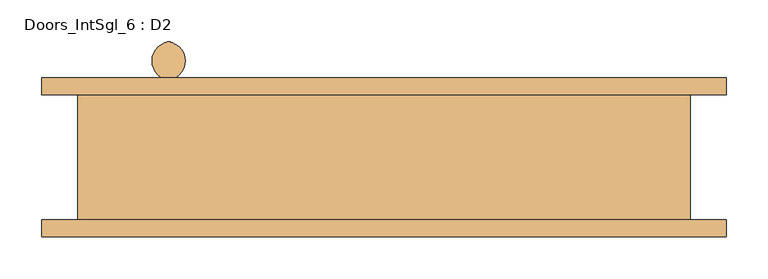
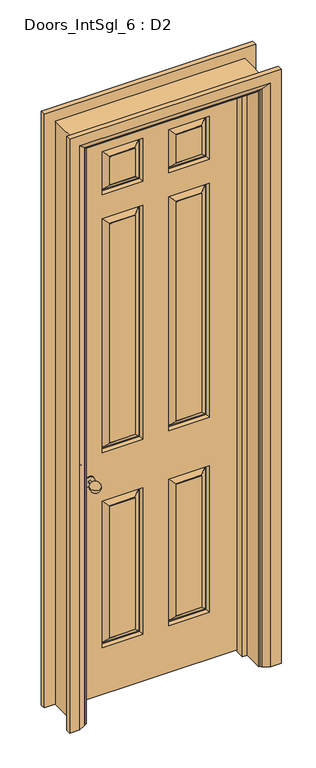
"""IFC4 building model written with IfcOpenShell, lengths in millimetres: door geometry, Doors_IntSgl_6 : D2."""

from ifc_helpers import new_model, si_unit, point, frame, origin, place, context, project, spatial, polyline, circle_curve, ellipse_curve, trimmed, outline, extrude, faceted_brep, source, transform, mapped, element, save
from ifc_brep_helpers import plane_surface, cylinder_surface, revolved_surface, advanced_brep


def doors_intsgl_6_d2_b603f254(model_context):
    return source(origin(), model_context, "Body", "SolidModel", [
        advanced_brep(
        [(-253.0, 18.0, 900.0), (-258.0, -26.437411, 900.0), (-263.0, 18.0, 900.0), (-263.0, 33.0, 900.0), (-253.0, 33.0, 900.0), (-278.0, 37.0, 900.0), (-238.0, 37.0, 900.0), (-278.0, 33.0, 900.0), (-238.0, 33.0, 900.0)],
        [
            (0, 1, circle_curve(frame((-261.1884862, -3.5786495, 900.0), z_axis=(0.0, 0.0, -1.0), x_axis=(0.0, 1.0, 0.0)), 23.0800654)),
            (1, 2, circle_curve(frame((-254.8115138, -3.5786495, 900.0), z_axis=(0.0, 0.0, -1.0), x_axis=(0.0, 1.0, 0.0)), 23.0800654)),
            (2, 0, circle_curve(frame((-258.0, 18.0, 900.0), z_axis=(0.0, -1.0, 0.0), x_axis=(-1.0, 0.0, 0.0)), 5.0)),
            (0, 2, circle_curve(frame((-258.0, 18.0, 900.0), z_axis=(0.0, -1.0, 0.0), x_axis=(-1.0, 0.0, 0.0)), 5.0)),
            (2, 3),
            (3, 4, circle_curve(frame((-258.0, 33.0, 900.0), z_axis=(0.0, -1.0, 0.0), x_axis=(-1.0, 0.0, 0.0)), 5.0)),
            (4, 0),
            (4, 3, circle_curve(frame((-258.0, 33.0, 900.0), z_axis=(0.0, -1.0, 0.0), x_axis=(-1.0, 0.0, 0.0)), 5.0)),
            (5, 6, circle_curve(frame((-258.0, 37.0, 900.0), z_axis=(0.0, 1.0, 0.0), x_axis=(1.0, 0.0, 0.0)), 20.0)),
            (6, 5, circle_curve(frame((-258.0, 37.0, 900.0), z_axis=(0.0, 1.0, 0.0), x_axis=(1.0, 0.0, 0.0)), 20.0)),
            (7, 8, circle_curve(frame((-258.0, 33.0, 900.0), z_axis=(0.0, -1.0, 0.0), x_axis=(1.0, 0.0, 0.0)), 20.0)),
            (8, 7, circle_curve(frame((-258.0, 33.0, 900.0), z_axis=(0.0, -1.0, 0.0), x_axis=(1.0, 0.0, 0.0)), 20.0)),
            (6, 8),
            (7, 5),
        ],
        [
            revolved_surface(trimmed(ellipse_curve(frame((-254.8115138, -3.5786495, 900.0), z_axis=(0.0, 0.0, -1.0), x_axis=(0.0, 1.0, 0.0)), 23.0800654, 23.0800654), [point((-258.0, -26.437411, 900.0))], [point((-263.0, 18.0, 900.0))], True, "CARTESIAN"), (-258.0, 33.0, 900.0), (0.0, 1.0, 0.0)),
            cylinder_surface(frame((-258.0, 33.0, 900.0), z_axis=(0.0, 1.0, 0.0), x_axis=(-1.0, 0.0, 0.0)), 5.0),
            plane_surface(frame((-238.0, 37.0, 900.0), z_axis=(0.0, 1.0, 0.0), x_axis=(0.0, 0.0, 1.0))),
            plane_surface(frame((-238.0, 33.0, 900.0), z_axis=(0.0, -1.0, 0.0), x_axis=(0.0, 0.0, -1.0))),
            cylinder_surface(frame((-258.0, 33.0, 900.0), z_axis=(0.0, 1.0, 0.0), x_axis=(1.0, 0.0, 0.0)), 20.0),
        ],
        [
            (0, [[1, 2, 3]]),
            (0, [[-1, 4, -2]]),
            (1, [[5, 6, 7, -3]]),
            (1, [[-7, 8, -5, -4]]),
            (2, [[9, 10]]),
            (3, [[11, 12], [-8, -6]]),
            (4, [[13, -11, 14, -10]]),
            (4, [[-14, -12, -13, -9]]),
        ],
    ),
        advanced_brep(
        [(-253.0, 94.0, 900.0), (-263.0, 94.0, 900.0), (-258.0, 138.437411, 900.0), (-253.0, 79.0, 900.0), (-263.0, 79.0, 900.0), (-278.0, 75.0, 900.0), (-238.0, 75.0, 900.0), (-278.0, 79.0, 900.0), (-238.0, 79.0, 900.0)],
        [
            (0, 1, circle_curve(frame((-258.0, 94.0, 900.0), z_axis=(0.0, 1.0, 0.0), x_axis=(-1.0, 0.0, 0.0)), 5.0)),
            (1, 2, circle_curve(frame((-254.8115138, 115.5786495, 900.0), z_axis=(0.0, 0.0, -1.0), x_axis=(0.0, -1.0, 0.0)), 23.0800654)),
            (2, 0, circle_curve(frame((-261.1884862, 115.5786495, 900.0), z_axis=(0.0, 0.0, -1.0), x_axis=(0.0, -1.0, 0.0)), 23.0800654)),
            (1, 0, circle_curve(frame((-258.0, 94.0, 900.0), z_axis=(0.0, 1.0, 0.0), x_axis=(-1.0, 0.0, 0.0)), 5.0)),
            (0, 3),
            (3, 4, circle_curve(frame((-258.0, 79.0, 900.0), z_axis=(0.0, 1.0, 0.0), x_axis=(-1.0, 0.0, 0.0)), 5.0)),
            (4, 1),
            (4, 3, circle_curve(frame((-258.0, 79.0, 900.0), z_axis=(0.0, 1.0, 0.0), x_axis=(-1.0, 0.0, 0.0)), 5.0)),
            (5, 6, circle_curve(frame((-258.0, 75.0, 900.0), z_axis=(0.0, -1.0, 0.0), x_axis=(1.0, 0.0, 0.0)), 20.0)),
            (6, 5, circle_curve(frame((-258.0, 75.0, 900.0), z_axis=(0.0, -1.0, 0.0), x_axis=(1.0, 0.0, 0.0)), 20.0)),
            (7, 8, circle_curve(frame((-258.0, 79.0, 900.0), z_axis=(0.0, 1.0, 0.0), x_axis=(1.0, 0.0, 0.0)), 20.0)),
            (8, 7, circle_curve(frame((-258.0, 79.0, 900.0), z_axis=(0.0, 1.0, 0.0), x_axis=(1.0, 0.0, 0.0)), 20.0)),
            (5, 7),
            (8, 6),
        ],
        [
            revolved_surface(trimmed(ellipse_curve(frame((-254.8115138, 115.5786495, 900.0), z_axis=(0.0, 0.0, 1.0), x_axis=(0.0, -1.0, 0.0)), 23.0800654, 23.0800654), [point((-258.0, 138.437411, 900.0))], [point((-263.0, 94.0, 900.0))], True, "CARTESIAN"), (-258.0, 79.0, 900.0), (0.0, -1.0, 0.0)),
            cylinder_surface(frame((-258.0, 79.0, 900.0), z_axis=(0.0, -1.0, 0.0), x_axis=(-1.0, 0.0, 0.0)), 5.0),
            plane_surface(frame((-238.0, 75.0, 900.0), z_axis=(0.0, -1.0, 0.0), x_axis=(0.0, 0.0, 1.0))),
            plane_surface(frame((-238.0, 79.0, 900.0), z_axis=(0.0, 1.0, 0.0), x_axis=(0.0, 0.0, -1.0))),
            cylinder_surface(frame((-258.0, 79.0, 900.0), z_axis=(0.0, -1.0, 0.0), x_axis=(1.0, 0.0, 0.0)), 20.0),
        ],
        [
            (0, [[1, 2, 3]]),
            (0, [[-2, 4, -3]]),
            (1, [[-1, 5, 6, 7]]),
            (1, [[-4, -7, 8, -5]]),
            (2, [[9, 10]]),
            (3, [[11, 12], [-6, -8]]),
            (4, [[-9, 13, -12, 14]]),
            (4, [[-10, -14, -11, -13]]),
        ],
    ),
        faceted_brep([(-333.0, 37.0, 2358.0), (-333.0, 37.0, 8.0), (333.0, 37.0, 8.0), (333.0, 37.0, 2358.0), (-50.0, 37.0, 800.0), (-50.0, 37.0, 200.0), (-208.0, 37.0, 200.0), (-208.0, 37.0, 800.0), (208.0, 37.0, 800.0), (208.0, 37.0, 200.0), (50.0, 37.0, 200.0), (50.0, 37.0, 800.0), (-50.0, 37.0, 1958.0), (-50.0, 37.0, 1000.0), (-208.0, 37.0, 1000.0), (-208.0, 37.0, 1958.0), (208.0, 37.0, 1958.0), (208.0, 37.0, 1000.0), (50.0, 37.0, 1000.0), (50.0, 37.0, 1958.0), (-50.0, 37.0, 2233.0), (-50.0, 37.0, 2058.0), (-208.0, 37.0, 2058.0), (-208.0, 37.0, 2233.0), (208.0, 37.0, 2233.0), (208.0, 37.0, 2058.0), (50.0, 37.0, 2058.0), (50.0, 37.0, 2233.0), (-80.0, 37.0, 230.0), (-80.0, 37.0, 770.0), (-178.0, 37.0, 770.0), (-178.0, 37.0, 230.0), (178.0, 37.0, 230.0), (178.0, 37.0, 770.0), (80.0, 37.0, 770.0), (80.0, 37.0, 230.0), (-80.0, 37.0, 1030.0), (-80.0, 37.0, 1928.0), (-178.0, 37.0, 1928.0), (-178.0, 37.0, 1030.0), (178.0, 37.0, 1030.0), (178.0, 37.0, 1928.0), (80.0, 37.0, 1928.0), (80.0, 37.0, 1030.0), (-80.0, 37.0, 2088.0), (-80.0, 37.0, 2203.0), (-178.0, 37.0, 2203.0), (-178.0, 37.0, 2088.0), (178.0, 37.0, 2088.0), (178.0, 37.0, 2203.0), (80.0, 37.0, 2203.0), (80.0, 37.0, 2088.0), (-333.0, 75.0, 2358.0), (333.0, 75.0, 2358.0), (333.0, 75.0, 8.0), (-333.0, 75.0, 8.0), (50.0, 75.0, 800.0), (50.0, 75.0, 200.0), (208.0, 75.0, 200.0), (208.0, 75.0, 800.0), (-208.0, 75.0, 800.0), (-208.0, 75.0, 200.0), (-50.0, 75.0, 200.0), (-50.0, 75.0, 800.0), (50.0, 75.0, 1958.0), (50.0, 75.0, 1000.0), (208.0, 75.0, 1000.0), (208.0, 75.0, 1958.0), (-208.0, 75.0, 1958.0), (-208.0, 75.0, 1000.0), (-50.0, 75.0, 1000.0), (-50.0, 75.0, 1958.0), (50.0, 75.0, 2233.0), (50.0, 75.0, 2058.0), (208.0, 75.0, 2058.0), (208.0, 75.0, 2233.0), (-208.0, 75.0, 2233.0), (-208.0, 75.0, 2058.0), (-50.0, 75.0, 2058.0), (-50.0, 75.0, 2233.0), (80.0, 75.0, 230.0), (80.0, 75.0, 770.0), (178.0, 75.0, 770.0), (178.0, 75.0, 230.0), (-178.0, 75.0, 230.0), (-178.0, 75.0, 770.0), (-80.0, 75.0, 770.0), (-80.0, 75.0, 230.0), (80.0, 75.0, 1030.0), (80.0, 75.0, 1928.0), (178.0, 75.0, 1928.0), (178.0, 75.0, 1030.0), (-178.0, 75.0, 1030.0), (-178.0, 75.0, 1928.0), (-80.0, 75.0, 1928.0), (-80.0, 75.0, 1030.0), (80.0, 75.0, 2088.0), (80.0, 75.0, 2203.0), (178.0, 75.0, 2203.0), (178.0, 75.0, 2088.0), (-178.0, 75.0, 2088.0), (-178.0, 75.0, 2203.0), (-80.0, 75.0, 2203.0), (-80.0, 75.0, 2088.0), (80.0, 74.0, 230.0), (80.0, 74.0, 770.0), (58.0, 60.0, 208.0), (58.0, 60.0, 792.0), (78.0, 74.0, 772.0), (78.0, 74.0, 228.0), (53.0, 60.0, 797.0), (53.0, 60.0, 203.0), (178.0, 74.0, 770.0), (200.0, 60.0, 792.0), (180.0, 74.0, 772.0), (205.0, 60.0, 797.0), (178.0, 74.0, 230.0), (200.0, 60.0, 208.0), (180.0, 74.0, 228.0), (205.0, 60.0, 203.0), (-178.0, 74.0, 230.0), (-178.0, 74.0, 770.0), (-200.0, 60.0, 208.0), (-200.0, 60.0, 792.0), (-180.0, 74.0, 772.0), (-180.0, 74.0, 228.0), (-205.0, 60.0, 797.0), (-205.0, 60.0, 203.0), (-80.0, 74.0, 770.0), (-58.0, 60.0, 792.0), (-78.0, 74.0, 772.0), (-53.0, 60.0, 797.0), (-80.0, 74.0, 230.0), (-58.0, 60.0, 208.0), (-78.0, 74.0, 228.0), (-53.0, 60.0, 203.0), (80.0, 74.0, 1030.0), (80.0, 74.0, 1928.0), (58.0, 60.0, 1008.0), (58.0, 60.0, 1950.0), (78.0, 74.0, 1930.0), (78.0, 74.0, 1028.0), (53.0, 60.0, 1955.0), (53.0, 60.0, 1003.0), (178.0, 74.0, 1928.0), (200.0, 60.0, 1950.0), (180.0, 74.0, 1930.0), (205.0, 60.0, 1955.0), (178.0, 74.0, 1030.0), (200.0, 60.0, 1008.0), (180.0, 74.0, 1028.0), (205.0, 60.0, 1003.0), (-178.0, 74.0, 1030.0), (-178.0, 74.0, 1928.0), (-200.0, 60.0, 1008.0), (-200.0, 60.0, 1950.0), (-180.0, 74.0, 1930.0), (-180.0, 74.0, 1028.0), (-205.0, 60.0, 1955.0), (-205.0, 60.0, 1003.0), (-80.0, 74.0, 1928.0), (-58.0, 60.0, 1950.0), (-78.0, 74.0, 1930.0), (-53.0, 60.0, 1955.0), (-80.0, 74.0, 1030.0), (-58.0, 60.0, 1008.0), (-78.0, 74.0, 1028.0), (-53.0, 60.0, 1003.0), (80.0, 74.0, 2088.0), (80.0, 74.0, 2203.0), (58.0, 60.0, 2066.0), (58.0, 60.0, 2225.0), (78.0, 74.0, 2205.0), (78.0, 74.0, 2086.0), (53.0, 60.0, 2230.0), (53.0, 60.0, 2061.0), (178.0, 74.0, 2203.0), (200.0, 60.0, 2225.0), (180.0, 74.0, 2205.0), (205.0, 60.0, 2230.0), (178.0, 74.0, 2088.0), (200.0, 60.0, 2066.0), (180.0, 74.0, 2086.0), (205.0, 60.0, 2061.0), (-178.0, 74.0, 2088.0), (-178.0, 74.0, 2203.0), (-200.0, 60.0, 2066.0), (-200.0, 60.0, 2225.0), (-180.0, 74.0, 2205.0), (-180.0, 74.0, 2086.0), (-205.0, 60.0, 2230.0), (-205.0, 60.0, 2061.0), (-80.0, 74.0, 2203.0), (-58.0, 60.0, 2225.0), (-78.0, 74.0, 2205.0), (-53.0, 60.0, 2230.0), (-80.0, 74.0, 2088.0), (-58.0, 60.0, 2066.0), (-78.0, 74.0, 2086.0), (-53.0, 60.0, 2061.0), (-80.0, 38.0, 230.0), (-80.0, 38.0, 770.0), (-58.0, 52.0, 208.0), (-58.0, 52.0, 792.0), (-78.0, 38.0, 772.0), (-78.0, 38.0, 228.0), (-53.0, 52.0, 797.0), (-53.0, 52.0, 203.0), (-178.0, 38.0, 770.0), (-200.0, 52.0, 792.0), (-180.0, 38.0, 772.0), (-205.0, 52.0, 797.0), (-178.0, 38.0, 230.0), (-200.0, 52.0, 208.0), (-180.0, 38.0, 228.0), (-205.0, 52.0, 203.0), (178.0, 38.0, 230.0), (178.0, 38.0, 770.0), (200.0, 52.0, 208.0), (200.0, 52.0, 792.0), (180.0, 38.0, 772.0), (180.0, 38.0, 228.0), (205.0, 52.0, 797.0), (205.0, 52.0, 203.0), (80.0, 38.0, 770.0), (58.0, 52.0, 792.0), (78.0, 38.0, 772.0), (53.0, 52.0, 797.0), (80.0, 38.0, 230.0), (58.0, 52.0, 208.0), (78.0, 38.0, 228.0), (53.0, 52.0, 203.0), (-80.0, 38.0, 1030.0), (-80.0, 38.0, 1928.0), (-58.0, 52.0, 1008.0), (-58.0, 52.0, 1950.0), (-78.0, 38.0, 1930.0), (-78.0, 38.0, 1028.0), (-53.0, 52.0, 1955.0), (-53.0, 52.0, 1003.0), (-178.0, 38.0, 1928.0), (-200.0, 52.0, 1950.0), (-180.0, 38.0, 1930.0), (-205.0, 52.0, 1955.0), (-178.0, 38.0, 1030.0), (-200.0, 52.0, 1008.0), (-180.0, 38.0, 1028.0), (-205.0, 52.0, 1003.0), (178.0, 38.0, 1030.0), (178.0, 38.0, 1928.0), (200.0, 52.0, 1008.0), (200.0, 52.0, 1950.0), (180.0, 38.0, 1930.0), (180.0, 38.0, 1028.0), (205.0, 52.0, 1955.0), (205.0, 52.0, 1003.0), (80.0, 38.0, 1928.0), (58.0, 52.0, 1950.0), (78.0, 38.0, 1930.0), (53.0, 52.0, 1955.0), (80.0, 38.0, 1030.0), (58.0, 52.0, 1008.0), (78.0, 38.0, 1028.0), (53.0, 52.0, 1003.0), (-80.0, 38.0, 2088.0), (-80.0, 38.0, 2203.0), (-58.0, 52.0, 2066.0), (-58.0, 52.0, 2225.0), (-78.0, 38.0, 2205.0), (-78.0, 38.0, 2086.0), (-53.0, 52.0, 2230.0), (-53.0, 52.0, 2061.0), (-178.0, 38.0, 2203.0), (-200.0, 52.0, 2225.0), (-180.0, 38.0, 2205.0), (-205.0, 52.0, 2230.0), (-178.0, 38.0, 2088.0), (-200.0, 52.0, 2066.0), (-180.0, 38.0, 2086.0), (-205.0, 52.0, 2061.0), (178.0, 38.0, 2088.0), (178.0, 38.0, 2203.0), (200.0, 52.0, 2066.0), (200.0, 52.0, 2225.0), (180.0, 38.0, 2205.0), (180.0, 38.0, 2086.0), (205.0, 52.0, 2230.0), (205.0, 52.0, 2061.0), (80.0, 38.0, 2203.0), (58.0, 52.0, 2225.0), (78.0, 38.0, 2205.0), (53.0, 52.0, 2230.0), (80.0, 38.0, 2088.0), (58.0, 52.0, 2066.0), (78.0, 38.0, 2086.0), (53.0, 52.0, 2061.0)], [[[0, 1, 2, 3], [4, 5, 6, 7], [8, 9, 10, 11], [12, 13, 14, 15], [16, 17, 18, 19], [20, 21, 22, 23], [24, 25, 26, 27]], [[28, 29, 30, 31]], [[32, 33, 34, 35]], [[36, 37, 38, 39]], [[40, 41, 42, 43]], [[44, 45, 46, 47]], [[48, 49, 50, 51]], [[52, 53, 54, 55], [56, 57, 58, 59], [60, 61, 62, 63], [64, 65, 66, 67], [68, 69, 70, 71], [72, 73, 74, 75], [76, 77, 78, 79]], [[80, 81, 82, 83]], [[84, 85, 86, 87]], [[88, 89, 90, 91]], [[92, 93, 94, 95]], [[96, 97, 98, 99]], [[100, 101, 102, 103]], [[1, 0, 52, 55]], [[2, 1, 55, 54]], [[3, 2, 54, 53]], [[0, 3, 53, 52]], [[104, 105, 81, 80]], [[106, 107, 108, 109]], [[56, 110, 111, 57]], [[81, 105, 112, 82]], [[108, 107, 113, 114]], [[110, 56, 59, 115]], [[82, 112, 116, 83]], [[114, 113, 117, 118]], [[115, 59, 58, 119]], [[104, 80, 83, 116]], [[109, 108, 114, 118], [105, 104, 116, 112]], [[106, 109, 118, 117]], [[111, 110, 115, 119], [107, 106, 117, 113]], [[57, 111, 119, 58]], [[120, 121, 85, 84]], [[122, 123, 124, 125]], [[60, 126, 127, 61]], [[85, 121, 128, 86]], [[124, 123, 129, 130]], [[126, 60, 63, 131]], [[86, 128, 132, 87]], [[130, 129, 133, 134]], [[131, 63, 62, 135]], [[120, 84, 87, 132]], [[125, 124, 130, 134], [121, 120, 132, 128]], [[122, 125, 134, 133]], [[127, 126, 131, 135], [123, 122, 133, 129]], [[61, 127, 135, 62]], [[136, 137, 89, 88]], [[138, 139, 140, 141]], [[64, 142, 143, 65]], [[89, 137, 144, 90]], [[140, 139, 145, 146]], [[142, 64, 67, 147]], [[90, 144, 148, 91]], [[146, 145, 149, 150]], [[147, 67, 66, 151]], [[136, 88, 91, 148]], [[141, 140, 146, 150], [137, 136, 148, 144]], [[138, 141, 150, 149]], [[143, 142, 147, 151], [139, 138, 149, 145]], [[65, 143, 151, 66]], [[152, 153, 93, 92]], [[154, 155, 156, 157]], [[68, 158, 159, 69]], [[93, 153, 160, 94]], [[156, 155, 161, 162]], [[158, 68, 71, 163]], [[94, 160, 164, 95]], [[162, 161, 165, 166]], [[163, 71, 70, 167]], [[152, 92, 95, 164]], [[157, 156, 162, 166], [153, 152, 164, 160]], [[154, 157, 166, 165]], [[159, 158, 163, 167], [155, 154, 165, 161]], [[69, 159, 167, 70]], [[168, 169, 97, 96]], [[170, 171, 172, 173]], [[72, 174, 175, 73]], [[97, 169, 176, 98]], [[172, 171, 177, 178]], [[174, 72, 75, 179]], [[98, 176, 180, 99]], [[178, 177, 181, 182]], [[179, 75, 74, 183]], [[168, 96, 99, 180]], [[173, 172, 178, 182], [169, 168, 180, 176]], [[170, 173, 182, 181]], [[175, 174, 179, 183], [171, 170, 181, 177]], [[73, 175, 183, 74]], [[184, 185, 101, 100]], [[186, 187, 188, 189]], [[76, 190, 191, 77]], [[101, 185, 192, 102]], [[188, 187, 193, 194]], [[190, 76, 79, 195]], [[102, 192, 196, 103]], [[194, 193, 197, 198]], [[195, 79, 78, 199]], [[184, 100, 103, 196]], [[189, 188, 194, 198], [185, 184, 196, 192]], [[186, 189, 198, 197]], [[191, 190, 195, 199], [187, 186, 197, 193]], [[77, 191, 199, 78]], [[200, 201, 29, 28]], [[202, 203, 204, 205]], [[4, 206, 207, 5]], [[29, 201, 208, 30]], [[204, 203, 209, 210]], [[206, 4, 7, 211]], [[30, 208, 212, 31]], [[210, 209, 213, 214]], [[211, 7, 6, 215]], [[200, 28, 31, 212]], [[205, 204, 210, 214], [201, 200, 212, 208]], [[202, 205, 214, 213]], [[207, 206, 211, 215], [203, 202, 213, 209]], [[5, 207, 215, 6]], [[216, 217, 33, 32]], [[218, 219, 220, 221]], [[8, 222, 223, 9]], [[33, 217, 224, 34]], [[220, 219, 225, 226]], [[222, 8, 11, 227]], [[34, 224, 228, 35]], [[226, 225, 229, 230]], [[227, 11, 10, 231]], [[216, 32, 35, 228]], [[221, 220, 226, 230], [217, 216, 228, 224]], [[218, 221, 230, 229]], [[223, 222, 227, 231], [219, 218, 229, 225]], [[9, 223, 231, 10]], [[232, 233, 37, 36]], [[234, 235, 236, 237]], [[12, 238, 239, 13]], [[37, 233, 240, 38]], [[236, 235, 241, 242]], [[238, 12, 15, 243]], [[38, 240, 244, 39]], [[242, 241, 245, 246]], [[243, 15, 14, 247]], [[232, 36, 39, 244]], [[237, 236, 242, 246], [233, 232, 244, 240]], [[234, 237, 246, 245]], [[239, 238, 243, 247], [235, 234, 245, 241]], [[13, 239, 247, 14]], [[248, 249, 41, 40]], [[250, 251, 252, 253]], [[16, 254, 255, 17]], [[41, 249, 256, 42]], [[252, 251, 257, 258]], [[254, 16, 19, 259]], [[42, 256, 260, 43]], [[258, 257, 261, 262]], [[259, 19, 18, 263]], [[248, 40, 43, 260]], [[253, 252, 258, 262], [249, 248, 260, 256]], [[250, 253, 262, 261]], [[255, 254, 259, 263], [251, 250, 261, 257]], [[17, 255, 263, 18]], [[264, 265, 45, 44]], [[266, 267, 268, 269]], [[20, 270, 271, 21]], [[45, 265, 272, 46]], [[268, 267, 273, 274]], [[270, 20, 23, 275]], [[46, 272, 276, 47]], [[274, 273, 277, 278]], [[275, 23, 22, 279]], [[264, 44, 47, 276]], [[269, 268, 274, 278], [265, 264, 276, 272]], [[266, 269, 278, 277]], [[271, 270, 275, 279], [267, 266, 277, 273]], [[21, 271, 279, 22]], [[280, 281, 49, 48]], [[282, 283, 284, 285]], [[24, 286, 287, 25]], [[49, 281, 288, 50]], [[284, 283, 289, 290]], [[286, 24, 27, 291]], [[50, 288, 292, 51]], [[290, 289, 293, 294]], [[291, 27, 26, 295]], [[280, 48, 51, 292]], [[285, 284, 290, 294], [281, 280, 292, 288]], [[282, 285, 294, 293]], [[287, 286, 291, 295], [283, 282, 293, 289]], [[25, 287, 295, 26]]]),
        faceted_brep([(-335.0, 75.0, 0.0), (-335.0, -75.0, 0.0), (-367.0, -75.0, 0.0), (-367.0, 75.0, 0.0), (-335.0, 75.0, 2360.0), (-335.0, -75.0, 2360.0), (-367.0, -75.0, 2392.0), (-367.0, 75.0, 2392.0), (335.0, 75.0, 0.0), (367.0, 75.0, 0.0), (367.0, -75.0, 0.0), (335.0, -75.0, 0.0), (335.0, 75.0, 2360.0), (367.0, 75.0, 2392.0), (367.0, -75.0, 2392.0), (335.0, -75.0, 2360.0)], [[[0, 1, 2, 3]], [[1, 0, 4, 5]], [[2, 1, 5, 6]], [[3, 2, 6, 7]], [[0, 3, 7, 4]], [[8, 9, 10, 11]], [[12, 13, 9, 8]], [[13, 14, 10, 9]], [[14, 15, 11, 10]], [[15, 12, 8, 11]], [[5, 4, 12, 15]], [[6, 5, 15, 14]], [[7, 6, 14, 13]], [[4, 7, 13, 12]]]),
        extrude(outline(polyline([(0.0, -335.0), (0.0, -316.0), (2341.0, -316.0), (2341.0, 316.0), (0.0, 316.0), (0.0, 335.0), (2360.0, 335.0), (2360.0, -335.0), (0.0, -335.0)])), frame((0.0, 3.0, 0.0), z_axis=(0.0, 1.0, 0.0), x_axis=(0.0, 0.0, 1.0)), (0.0, 0.0, 1.0), 32.0),
        advanced_brep(
        [(-410.0, -95.0, 0.0), (-410.0, -75.0, 0.0), (-340.0, -75.0, 0.0), (-344.0, -81.0, 0.0), (-370.0, -95.0, 0.0), (-410.0, -95.0, 2435.0), (-410.0, -75.0, 2435.0), (410.0, -75.0, 2435.0), (410.0, -75.0, 0.0), (340.0, -75.0, 0.0), (340.0, -75.0, 2365.0), (-340.0, -75.0, 2365.0), (-344.0, -81.0, 2369.0), (-370.0, -95.0, 2395.0), (370.0, -95.0, 2395.0), (370.0, -95.0, 0.0), (410.0, -95.0, 0.0), (410.0, -95.0, 2435.0), (344.0, -81.0, 0.0), (344.0, -81.0, 2369.0)],
        [
            (0, 1),
            (1, 2),
            (2, 3, circle_curve(frame((-348.0, -74.0, 0.0), z_axis=(0.0, 0.0, -1.0), x_axis=(-1.0, 0.0, 0.0)), 8.0622577)),
            (3, 4),
            (4, 0),
            (0, 5),
            (5, 6),
            (6, 1),
            (6, 7),
            (7, 8),
            (8, 9),
            (9, 10),
            (10, 11),
            (11, 2),
            (11, 12, ellipse_curve(frame((-348.0, -74.0, 2373.0), z_axis=(-0.7071067811865475, 0.0, -0.7071067811865475), x_axis=(0.7071067811865474, 0.0, -0.7071067811865476)), 11.4017543, 8.0622577)),
            (12, 3),
            (12, 13),
            (13, 4),
            (13, 14),
            (14, 15),
            (15, 16),
            (16, 17),
            (17, 5),
            (7, 17),
            (16, 8),
            (15, 18),
            (18, 9, circle_curve(frame((348.0, -74.0, 0.0), z_axis=(0.0, 0.0, -1.0), x_axis=(1.0, 0.0, 0.0)), 8.0622577)),
            (19, 10, ellipse_curve(frame((348.0, -74.0, 2373.0), z_axis=(0.7071067811865475, 0.0, -0.7071067811865475), x_axis=(0.7071067811865474, 0.0, 0.7071067811865476)), 11.4017543, 8.0622577)),
            (18, 19),
            (14, 19),
            (19, 12),
        ],
        [
            plane_surface(frame((-340.0, -75.0, 0.0), z_axis=(0.0, 0.0, -1.0), x_axis=(0.0, -1.0, 0.0))),
            plane_surface(frame((-410.0, -95.0, 0.0), z_axis=(-1.0, 0.0, 0.0), x_axis=(0.0, 0.0, 1.0))),
            plane_surface(frame((-410.0, -75.0, 0.0), z_axis=(0.0, 1.0, 0.0), x_axis=(0.0, 0.0, 1.0))),
            cylinder_surface(frame((-348.0, -74.0, 0.0), z_axis=(0.0, 0.0, -1.0), x_axis=(-1.0, 0.0, 0.0)), 8.0622577),
            plane_surface(frame((-344.0, -81.0, 0.0), z_axis=(0.4740998230350183, -0.8804710999221749, 0.0), x_axis=(0.0, 0.0, 1.0))),
            plane_surface(frame((-370.0, -95.0, 0.0), z_axis=(0.0, -1.0, 0.0), x_axis=(0.0, 0.0, 1.0))),
            plane_surface(frame((410.0, -95.0, 2435.0), z_axis=(1.0, 0.0, 0.0), x_axis=(0.0, 0.0, -1.0))),
            plane_surface(frame((340.0, -75.0, 0.0), z_axis=(0.0, 0.0, -1.0), x_axis=(0.0, -1.0, 0.0))),
            cylinder_surface(frame((348.0, -74.0, 2365.0), z_axis=(0.0, 0.0, 1.0), x_axis=(1.0, 0.0, 0.0)), 8.0622577),
            plane_surface(frame((344.0, -81.0, 2369.0), z_axis=(-0.4740998230350183, -0.8804710999221749, 0.0), x_axis=(0.0, 0.0, -1.0))),
            plane_surface(frame((-410.0, -95.0, 2435.0), z_axis=(0.0, 0.0, 1.0), x_axis=(1.0, 0.0, 0.0))),
            cylinder_surface(frame((-340.0, -74.0, 2373.0), z_axis=(-1.0, 0.0, 0.0), x_axis=(0.0, 0.0, 1.0)), 8.0622577),
            plane_surface(frame((-344.0, -81.0, 2369.0), z_axis=(0.0, -0.8804710999221749, -0.4740998230350183), x_axis=(1.0, 0.0, 0.0))),
        ],
        [
            (0, [[1, 2, 3, 4, 5]]),
            (1, [[-1, 6, 7, 8]]),
            (2, [[-2, -8, 9, 10, 11, 12, 13, 14]]),
            (3, [[-3, -14, 15, 16]]),
            (4, [[-4, -16, 17, 18]]),
            (5, [[-5, -18, 19, 20, 21, 22, 23, -6]]),
            (6, [[24, -22, 25, -10]]),
            (7, [[-21, 26, 27, -11, -25]]),
            (8, [[28, -12, -27, 29]]),
            (9, [[30, -29, -26, -20]]),
            (10, [[-7, -23, -24, -9]]),
            (11, [[-15, -13, -28, 31]]),
            (12, [[-17, -31, -30, -19]]),
        ],
    ),
        advanced_brep(
        [(410.0, 95.0, 0.0), (410.0, 75.0, 0.0), (340.0, 75.0, 0.0), (344.0, 81.0, 0.0), (370.0, 95.0, 0.0), (410.0, 95.0, 2435.0), (410.0, 75.0, 2435.0), (-410.0, 75.0, 2435.0), (-410.0, 75.0, 0.0), (-340.0, 75.0, 0.0), (-340.0, 75.0, 2365.0), (340.0, 75.0, 2365.0), (344.0, 81.0, 2369.0), (370.0, 95.0, 2395.0), (-370.0, 95.0, 2395.0), (-370.0, 95.0, 0.0), (-410.0, 95.0, 0.0), (-410.0, 95.0, 2435.0), (-344.0, 81.0, 0.0), (-344.0, 81.0, 2369.0)],
        [
            (0, 1),
            (1, 2),
            (2, 3, circle_curve(frame((348.0, 74.0, 0.0), z_axis=(0.0, 0.0, -1.0), x_axis=(1.0, 0.0, 0.0)), 8.0622577)),
            (3, 4),
            (4, 0),
            (0, 5),
            (5, 6),
            (6, 1),
            (6, 7),
            (7, 8),
            (8, 9),
            (9, 10),
            (10, 11),
            (11, 2),
            (11, 12, ellipse_curve(frame((348.0, 74.0, 2373.0), z_axis=(0.7071067811865475, 0.0, -0.7071067811865475), x_axis=(-0.7071067811865474, 0.0, -0.7071067811865476)), 11.4017543, 8.0622577)),
            (12, 3),
            (12, 13),
            (13, 4),
            (13, 14),
            (14, 15),
            (15, 16),
            (16, 17),
            (17, 5),
            (7, 17),
            (16, 8),
            (15, 18),
            (18, 9, circle_curve(frame((-348.0, 74.0, 0.0), z_axis=(0.0, 0.0, -1.0), x_axis=(-1.0, 0.0, 0.0)), 8.0622577)),
            (19, 10, ellipse_curve(frame((-348.0, 74.0, 2373.0), z_axis=(-0.7071067811865475, 0.0, -0.7071067811865475), x_axis=(-0.7071067811865474, 0.0, 0.7071067811865476)), 11.4017543, 8.0622577)),
            (18, 19),
            (14, 19),
            (19, 12),
        ],
        [
            plane_surface(frame((340.0, 75.0, 0.0), z_axis=(0.0, 0.0, -1.0), x_axis=(0.0, 1.0, 0.0))),
            plane_surface(frame((410.0, 95.0, 0.0), z_axis=(1.0, 0.0, 0.0), x_axis=(0.0, 0.0, 1.0))),
            plane_surface(frame((410.0, 75.0, 0.0), z_axis=(0.0, -1.0, 0.0), x_axis=(0.0, 0.0, 1.0))),
            cylinder_surface(frame((348.0, 74.0, 0.0), z_axis=(0.0, 0.0, -1.0), x_axis=(1.0, 0.0, 0.0)), 8.0622577),
            plane_surface(frame((344.0, 81.0, 0.0), z_axis=(-0.4740998230350183, 0.8804710999221749, 0.0), x_axis=(0.0, 0.0, 1.0))),
            plane_surface(frame((370.0, 95.0, 0.0), z_axis=(0.0, 1.0, 0.0), x_axis=(0.0, 0.0, 1.0))),
            plane_surface(frame((-410.0, 95.0, 2435.0), z_axis=(-1.0, 0.0, 0.0), x_axis=(0.0, 0.0, -1.0))),
            plane_surface(frame((-340.0, 75.0, 0.0), z_axis=(0.0, 0.0, -1.0), x_axis=(0.0, 1.0, 0.0))),
            cylinder_surface(frame((-348.0, 74.0, 2365.0), z_axis=(0.0, 0.0, 1.0), x_axis=(-1.0, 0.0, 0.0)), 8.0622577),
            plane_surface(frame((-344.0, 81.0, 2369.0), z_axis=(0.4740998230350183, 0.8804710999221749, 0.0), x_axis=(0.0, 0.0, -1.0))),
            plane_surface(frame((410.0, 95.0, 2435.0), z_axis=(0.0, 0.0, 1.0), x_axis=(-1.0, 0.0, 0.0))),
            cylinder_surface(frame((340.0, 74.0, 2373.0), z_axis=(1.0, 0.0, 0.0), x_axis=(0.0, 0.0, 1.0)), 8.0622577),
            plane_surface(frame((344.0, 81.0, 2369.0), z_axis=(0.0, 0.8804710999221749, -0.4740998230350183), x_axis=(-1.0, 0.0, 0.0))),
        ],
        [
            (0, [[1, 2, 3, 4, 5]]),
            (1, [[-1, 6, 7, 8]]),
            (2, [[-2, -8, 9, 10, 11, 12, 13, 14]]),
            (3, [[-3, -14, 15, 16]]),
            (4, [[-4, -16, 17, 18]]),
            (5, [[-5, -18, 19, 20, 21, 22, 23, -6]]),
            (6, [[24, -22, 25, -10]]),
            (7, [[-21, 26, 27, -11, -25]]),
            (8, [[28, -12, -27, 29]]),
            (9, [[30, -29, -26, -20]]),
            (10, [[-7, -23, -24, -9]]),
            (11, [[-15, -13, -28, 31]]),
            (12, [[-17, -31, -30, -19]]),
        ],
    ),
    ])


if __name__ == "__main__":
    model = new_model("IFC4")
    model_context = context("Model", 3, world=origin())
    ifc_project = project(units=[si_unit("LENGTHUNIT", "METRE", prefix="MILLI")], contexts=[model_context])
    site = spatial("IfcSite", under=ifc_project)
    building = spatial("IfcBuilding", under=site)
    placement = place(None, origin())
    doors_intsgl_6_d2_shape = doors_intsgl_6_d2_b603f254(model_context)
    element("IfcDoor", 1, ObjectType="Doors_IntSgl_6 : D2", at=placement, inside=building, context=model_context, shape_type="MappedRepresentation", body=[
        mapped(doors_intsgl_6_d2_shape, transform((0.0, 0.0, 0.0), x_axis=(1.0, 0.0, 0.0), y_axis=(0.0, 1.0, 0.0), z_axis=(0.0, 0.0, 1.0))),
    ])
    save(model, "model.ifc")

# Revit data of these elements
# Type "Doors_IntSgl_6 : D2"
#   Type Mark = "50"
#   Type Comments = "Internal Single"
#   Operation = "SingleSwingRight"
#   Construction Type Id = "MDOOR"
#   Manufacturer = "Revit"
#   Keynote = "L20"
#   Description = "Internal Single Door"
#   Analytic Construction = "Metal"
#   UnderCut = 8 mm
#   Tolerance = 2 mm
#   Thickness = 38 mm
#   Structural Tolerance = 8 mm
#   StopDepth = 32 mm
#   Stop Thickness = 19 mm
#   Stile Top Rail = 125 mm
#   Stile Shutting = 125 mm
#   Stile Muntin Rail = 100 mm
#   Stile Lock Rail = 200 mm
#   Stile Intermediate/Frieze = 100 mm
#   Stile Hanging = 125 mm
#   Stile Bottom Rail = 200 mm
#   Rough Width = 750 mm
#   Rough Height = 2400 mm
#   Height to Top Lock Rail = 1000 mm
#   Heat Transfer Coefficient (U) = 3.7021 W/(m²·K)
#   Handle Z Distance = 900 mm
#   Handle X Distance = 75 mm
#   Frame Thickness = 32 mm
#   Door Panel Width = 666 mm
#   Height = 2400 mm
#   Width = 750 mm
#   Door Panel Thickness = 38 mm
#   Door Panel Offset = 0 mm
#   Door Panel Height = 2350 mm
#   Architrave Setback = 5 mm
#   Vis - Ironmongery = yes
#   Define Thermal Properties by = 1
#   Material Ironmongery = Door - Handle
#   Material Frame = Door - Frame/Mullion
#   Material Door = Door - Panel
#   Material Architrave = Door - Architrave
#   Visual Light Transmittance = 0
#   Solar Heat Gain Coefficient = 0
#   Function = (empty or 0)
#   Wall Closure = (empty or 0)
# Element 1 (IfcDoor, "Doors_IntSgl_6 : D2")
#   Materials on its faces: "Door - Panel", "Door - Architrave", "Door - Frame/Mullion", "Door - Handle"
# Materials
#   "Door - Handle": colour RGB 247 247 247, transparency 0
#   "Door - Frame/Mullion": class "Wood", colour RGB 212 179 113, transparency 0
#   "Door - Panel": class "Wood", colour RGB 154 90 5, transparency 0
#   "Door - Architrave": class "Wood", colour RGB 154 90 5, transparency 0
